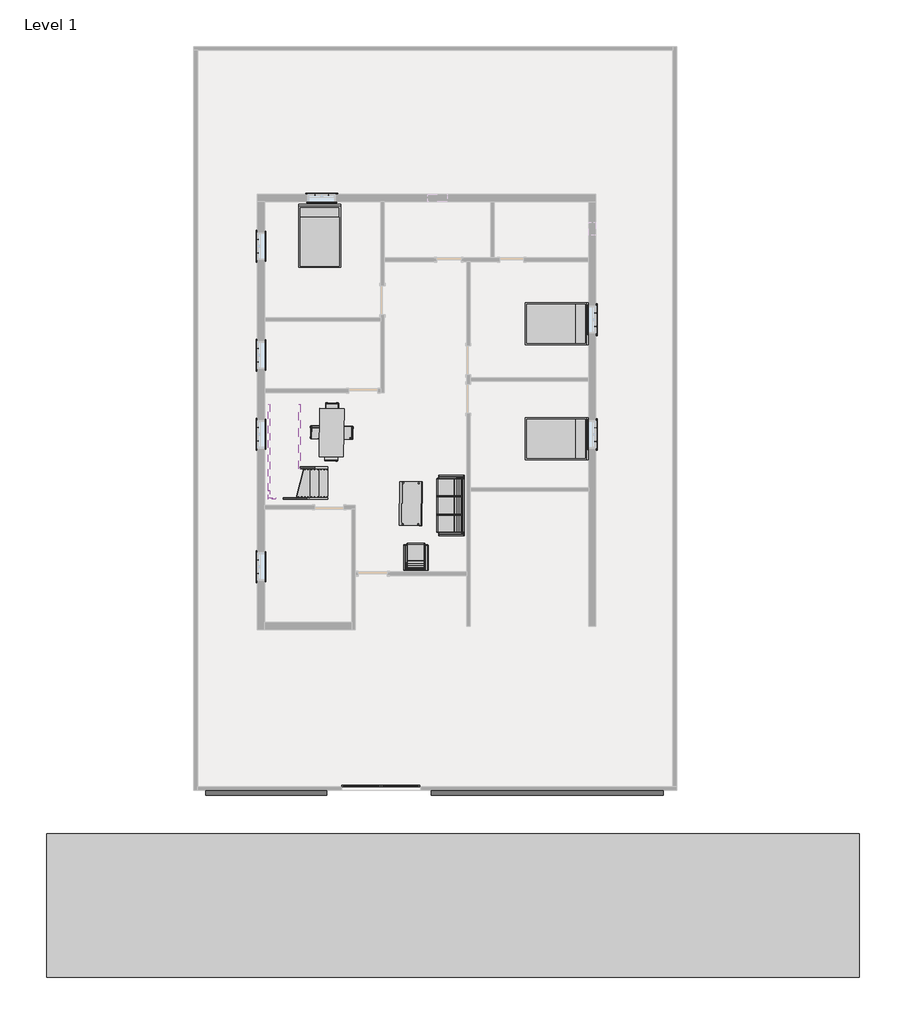
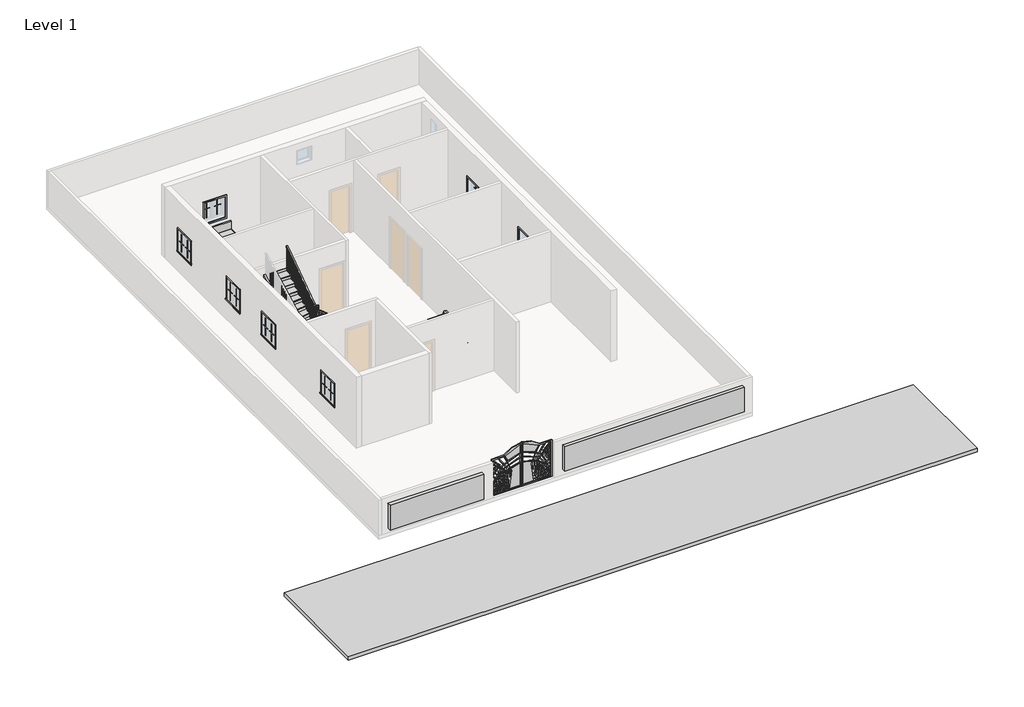
# One storey, part 2 of 2: 32 proxies, 6 furniture elements, 6 members, 1 railing, 1 stair flight.
"""IFC4 building model written with IfcOpenShell, lengths in millimetres."""

from ifc_helpers import new_model, si_unit, frame, origin, place, context, project, spatial, polyline, outline, extrude, faceted_brep, transform, mapped, element, save
from components import generic_models_6bc30956, generic_models_1_generic_models_1_70afe8e7, generic_models_2_generic_models_2_4f75562f, modern_coffee_table_17989_modern_coffee_table_17989_d3a860c8, muntin_pattern_2x2_muntin_pattern_2x2_b3fe6957, muntin_pattern_2x2_muntin_pattern_2x2_3e0ecaf2, trim_window_exterior_flat_with_sill_41619996, trim_window_interior_flat_picture_frame_51c85655, furniture_2fc85b74, furniture_29a9adb8, furniture_57072a26, furniture_f28dd14e, furniture_402a1f5e, bed_17739_bed_17739_15c61121, dining_table_w_chairs_11374_0cdfc61b, stair_flight_c47d8ec9

model = new_model("IFC4")

# Units and contexts
model_context = context("Model", 3, world=origin())
ifc_project = project(units=[si_unit("LENGTHUNIT", "METRE", prefix="MILLI")], contexts=[model_context])

# Site, building, storey
site = spatial("IfcSite", under=ifc_project)
building = spatial("IfcBuilding", under=site)
storey = spatial("IfcBuildingStorey", under=building, Name="Level 1", Elevation=0.0)

# Proxies
placement = place(None, origin())
generic_models_shape = generic_models_6bc30956(model_context)
element("IfcBuildingElementProxy", 1, Name="Generic Models", at=placement, inside=storey, context=model_context, shape_type="MappedRepresentation", body=[
    mapped(generic_models_shape, transform((-2704.2599931, -11222.4732708, 0.0), x_axis=(1.0, 0.0, 0.0), y_axis=(0.0, 1.0, 0.0), z_axis=(0.0, 0.0, 1.0))),
])
generic_models_1_generic_models_1_shape = generic_models_1_generic_models_1_70afe8e7(model_context)
element("IfcBuildingElementProxy", 2, Name="Generic Models 1 : Generic Models 1", ObjectType="Generic Models 1 : Generic Models 1", at=placement, inside=storey, context=model_context, shape_type="MappedRepresentation", body=[
    mapped(generic_models_1_generic_models_1_shape, transform((0.0, 0.0, 0.0), x_axis=(1.0, 0.0, 0.0), y_axis=(0.0, 1.0, 0.0), z_axis=(0.0, 0.0, 1.0))),
])
generic_models_2_generic_models_2_shape = generic_models_2_generic_models_2_4f75562f(model_context)
element("IfcBuildingElementProxy", 3, Name="Generic Models 2 : Generic Models 2", ObjectType="Generic Models 2 : Generic Models 2", at=placement, inside=storey, context=model_context, shape_type="MappedRepresentation", body=[
    mapped(generic_models_2_generic_models_2_shape, transform((0.0, 0.0, 0.0), x_axis=(1.0, 0.0, 0.0), y_axis=(0.0, 1.0, 0.0), z_axis=(0.0, 0.0, 1.0))),
])
modern_coffee_table_17989_modern_coffee_table_17989_shape = modern_coffee_table_17989_modern_coffee_table_17989_d3a860c8(model_context)
element("IfcBuildingElementProxy", 4, Name="Modern_Coffee_Table_17989 : Modern_Coffee_Table_17989", ObjectType="Modern_Coffee_Table_17989 : Modern_Coffee_Table_17989", at=placement, inside=storey, context=model_context, shape_type="MappedRepresentation", body=[
    mapped(modern_coffee_table_17989_modern_coffee_table_17989_shape, transform((-2106.8718825, -2116.758017, 0.0), x_axis=(0.012591066442684793, 0.9999207293810025, 0.0), y_axis=(-0.9999207293810025, 0.012591066442684793, 0.0), z_axis=(0.0, 0.0, 1.0))),
])
muntin_pattern_2x2_muntin_pattern_2x2_shape = muntin_pattern_2x2_muntin_pattern_2x2_b3fe6957(model_context)
element("IfcBuildingElementProxy", 5, Name="Muntin Pattern_2x2 : Muntin Pattern_2x2", ObjectType="Muntin Pattern_2x2 : Muntin Pattern_2x2", at=placement, inside=storey, context=model_context, shape_type="MappedRepresentation", body=[
    mapped(muntin_pattern_2x2_muntin_pattern_2x2_shape, transform((-4775.9474931, 7386.6685985, 984.25), x_axis=(1.0, 0.0, 0.0), y_axis=(0.0, 1.0, 0.0), z_axis=(0.0, 0.0, 1.0))),
])
element("IfcBuildingElementProxy", 6, Name="Muntin Pattern_2x2 : Muntin Pattern_2x2", ObjectType="Muntin Pattern_2x2 : Muntin Pattern_2x2", at=placement, inside=storey, context=model_context, shape_type="MappedRepresentation", body=[
    mapped(muntin_pattern_2x2_muntin_pattern_2x2_shape, transform((4068.0150069, 3660.8060985, 984.25), x_axis=(0.0, -1.0, 0.0), y_axis=(1.0, 0.0, 0.0), z_axis=(0.0, 0.0, 1.0))),
])
element("IfcBuildingElementProxy", 7, Name="Muntin Pattern_2x2 : Muntin Pattern_2x2", ObjectType="Muntin Pattern_2x2 : Muntin Pattern_2x2", at=placement, inside=storey, context=model_context, shape_type="MappedRepresentation", body=[
    mapped(muntin_pattern_2x2_muntin_pattern_2x2_shape, transform((4068.0150069, 40.9802908, 984.25), x_axis=(0.0, -1.0, 0.0), y_axis=(1.0, 0.0, 0.0), z_axis=(0.0, 0.0, 1.0))),
])
element("IfcBuildingElementProxy", 8, Name="Muntin Pattern_2x2 : Muntin Pattern_2x2", ObjectType="Muntin Pattern_2x2 : Muntin Pattern_2x2", at=placement, inside=storey, context=model_context, shape_type="MappedRepresentation", body=[
    mapped(muntin_pattern_2x2_muntin_pattern_2x2_shape, transform((-6580.9349931, 2114.5810985, 984.25), x_axis=(0.0, 1.0, 0.0), y_axis=(-1.0, 0.0, 0.0), z_axis=(0.0, 0.0, 1.0))),
])
element("IfcBuildingElementProxy", 9, Name="Muntin Pattern_2x2 : Muntin Pattern_2x2", ObjectType="Muntin Pattern_2x2 : Muntin Pattern_2x2", at=placement, inside=storey, context=model_context, shape_type="MappedRepresentation", body=[
    mapped(muntin_pattern_2x2_muntin_pattern_2x2_shape, transform((-6580.9349931, 5543.5810985, 984.25), x_axis=(0.0, 1.0, 0.0), y_axis=(-1.0, 0.0, 0.0), z_axis=(0.0, 0.0, 1.0))),
])
element("IfcBuildingElementProxy", 10, Name="Muntin Pattern_2x2 : Muntin Pattern_2x2", ObjectType="Muntin Pattern_2x2 : Muntin Pattern_2x2", at=placement, inside=storey, context=model_context, shape_type="MappedRepresentation", body=[
    mapped(muntin_pattern_2x2_muntin_pattern_2x2_shape, transform((-6580.9349931, -4549.7439015, 984.25), x_axis=(0.0, 1.0, 0.0), y_axis=(-1.0, 0.0, 0.0), z_axis=(0.0, 0.0, 1.0))),
])
element("IfcBuildingElementProxy", 11, Name="Muntin Pattern_2x2 : Muntin Pattern_2x2", ObjectType="Muntin Pattern_2x2 : Muntin Pattern_2x2", at=placement, inside=storey, context=model_context, shape_type="MappedRepresentation", body=[
    mapped(muntin_pattern_2x2_muntin_pattern_2x2_shape, transform((-6580.9349931, -380.9689015, 984.25), x_axis=(0.0, 1.0, 0.0), y_axis=(-1.0, 0.0, 0.0), z_axis=(0.0, 0.0, 1.0))),
])
muntin_pattern_2x2_muntin_pattern_2x2_2_shape = muntin_pattern_2x2_muntin_pattern_2x2_3e0ecaf2(model_context)
element("IfcBuildingElementProxy", 12, Name="Muntin Pattern_2x2 : Muntin Pattern_2x2", ObjectType="Muntin Pattern_2x2 : Muntin Pattern_2x2", at=placement, inside=storey, context=model_context, shape_type="MappedRepresentation", body=[
    mapped(muntin_pattern_2x2_muntin_pattern_2x2_2_shape, transform((-4347.3224931, 7386.6685985, 984.25), x_axis=(-1.0, 0.0, 0.0), y_axis=(0.0, -1.0, 0.0), z_axis=(0.0, 0.0, 1.0))),
])
element("IfcBuildingElementProxy", 13, Name="Muntin Pattern_2x2 : Muntin Pattern_2x2", ObjectType="Muntin Pattern_2x2 : Muntin Pattern_2x2", at=placement, inside=storey, context=model_context, shape_type="MappedRepresentation", body=[
    mapped(muntin_pattern_2x2_muntin_pattern_2x2_2_shape, transform((4068.0150069, 3232.1810985, 984.25), x_axis=(0.0, 1.0, 0.0), y_axis=(-1.0, 0.0, 0.0), z_axis=(0.0, 0.0, 1.0))),
])
element("IfcBuildingElementProxy", 14, Name="Muntin Pattern_2x2 : Muntin Pattern_2x2", ObjectType="Muntin Pattern_2x2 : Muntin Pattern_2x2", at=placement, inside=storey, context=model_context, shape_type="MappedRepresentation", body=[
    mapped(muntin_pattern_2x2_muntin_pattern_2x2_2_shape, transform((4068.0150069, -387.6447092, 984.25), x_axis=(0.0, 1.0, 0.0), y_axis=(-1.0, 0.0, 0.0), z_axis=(0.0, 0.0, 1.0))),
])
element("IfcBuildingElementProxy", 15, Name="Muntin Pattern_2x2 : Muntin Pattern_2x2", ObjectType="Muntin Pattern_2x2 : Muntin Pattern_2x2", at=placement, inside=storey, context=model_context, shape_type="MappedRepresentation", body=[
    mapped(muntin_pattern_2x2_muntin_pattern_2x2_2_shape, transform((-6580.9349931, 2543.2060985, 984.25), x_axis=(0.0, -1.0, 0.0), y_axis=(1.0, 0.0, 0.0), z_axis=(0.0, 0.0, 1.0))),
])
element("IfcBuildingElementProxy", 16, Name="Muntin Pattern_2x2 : Muntin Pattern_2x2", ObjectType="Muntin Pattern_2x2 : Muntin Pattern_2x2", at=placement, inside=storey, context=model_context, shape_type="MappedRepresentation", body=[
    mapped(muntin_pattern_2x2_muntin_pattern_2x2_2_shape, transform((-6580.9349931, 5972.2060985, 984.25), x_axis=(0.0, -1.0, 0.0), y_axis=(1.0, 0.0, 0.0), z_axis=(0.0, 0.0, 1.0))),
])
element("IfcBuildingElementProxy", 17, Name="Muntin Pattern_2x2 : Muntin Pattern_2x2", ObjectType="Muntin Pattern_2x2 : Muntin Pattern_2x2", at=placement, inside=storey, context=model_context, shape_type="MappedRepresentation", body=[
    mapped(muntin_pattern_2x2_muntin_pattern_2x2_2_shape, transform((-6580.9349931, -4121.1189015, 984.25), x_axis=(0.0, -1.0, 0.0), y_axis=(1.0, 0.0, 0.0), z_axis=(0.0, 0.0, 1.0))),
])
element("IfcBuildingElementProxy", 18, Name="Muntin Pattern_2x2 : Muntin Pattern_2x2", ObjectType="Muntin Pattern_2x2 : Muntin Pattern_2x2", at=placement, inside=storey, context=model_context, shape_type="MappedRepresentation", body=[
    mapped(muntin_pattern_2x2_muntin_pattern_2x2_2_shape, transform((-6580.9349931, 47.6560985, 984.25), x_axis=(0.0, -1.0, 0.0), y_axis=(1.0, 0.0, 0.0), z_axis=(0.0, 0.0, 1.0))),
])
trim_window_exterior_flat_with_sill_shape = trim_window_exterior_flat_with_sill_41619996(model_context)
element("IfcBuildingElementProxy", 19, Name="Trim-Window-Exterior-Flat : with Sill", ObjectType="Trim-Window-Exterior-Flat : with Sill", at=placement, inside=storey, context=model_context, shape_type="MappedRepresentation", body=[
    mapped(trim_window_exterior_flat_with_sill_shape, transform((-4561.6349931, 7396.1935985, 1828.8), x_axis=(-1.0, 0.0, 0.0), y_axis=(0.0, 0.0, 1.0), z_axis=(0.0, 1.0, 0.0))),
])
element("IfcBuildingElementProxy", 20, Name="Trim-Window-Exterior-Flat : with Sill", ObjectType="Trim-Window-Exterior-Flat : with Sill", at=placement, inside=storey, context=model_context, shape_type="MappedRepresentation", body=[
    mapped(trim_window_exterior_flat_with_sill_shape, transform((4077.5400069, 3446.4935985, 1828.8), x_axis=(0.0, 1.0, 0.0), y_axis=(0.0, 0.0, 1.0), z_axis=(1.0, 0.0, 0.0))),
])
element("IfcBuildingElementProxy", 21, Name="Trim-Window-Exterior-Flat : with Sill", ObjectType="Trim-Window-Exterior-Flat : with Sill", at=placement, inside=storey, context=model_context, shape_type="MappedRepresentation", body=[
    mapped(trim_window_exterior_flat_with_sill_shape, transform((4077.5400069, -173.3322092, 1828.8), x_axis=(0.0, 1.0, 0.0), y_axis=(0.0, 0.0, 1.0), z_axis=(1.0, 0.0, 0.0))),
])
element("IfcBuildingElementProxy", 22, Name="Trim-Window-Exterior-Flat : with Sill", ObjectType="Trim-Window-Exterior-Flat : with Sill", at=placement, inside=storey, context=model_context, shape_type="MappedRepresentation", body=[
    mapped(trim_window_exterior_flat_with_sill_shape, transform((-6590.4599931, 2328.8935985, 1828.8), x_axis=(0.0, -1.0, 0.0), y_axis=(0.0, 0.0, 1.0), z_axis=(-1.0, 0.0, 0.0))),
])
element("IfcBuildingElementProxy", 23, Name="Trim-Window-Exterior-Flat : with Sill", ObjectType="Trim-Window-Exterior-Flat : with Sill", at=placement, inside=storey, context=model_context, shape_type="MappedRepresentation", body=[
    mapped(trim_window_exterior_flat_with_sill_shape, transform((-6590.4599931, 5757.8935985, 1828.8), x_axis=(0.0, -1.0, 0.0), y_axis=(0.0, 0.0, 1.0), z_axis=(-1.0, 0.0, 0.0))),
])
element("IfcBuildingElementProxy", 24, Name="Trim-Window-Exterior-Flat : with Sill", ObjectType="Trim-Window-Exterior-Flat : with Sill", at=placement, inside=storey, context=model_context, shape_type="MappedRepresentation", body=[
    mapped(trim_window_exterior_flat_with_sill_shape, transform((-6590.4599931, -4335.4314015, 1828.8), x_axis=(0.0, -1.0, 0.0), y_axis=(0.0, 0.0, 1.0), z_axis=(-1.0, 0.0, 0.0))),
])
element("IfcBuildingElementProxy", 25, Name="Trim-Window-Exterior-Flat : with Sill", ObjectType="Trim-Window-Exterior-Flat : with Sill", at=placement, inside=storey, context=model_context, shape_type="MappedRepresentation", body=[
    mapped(trim_window_exterior_flat_with_sill_shape, transform((-6590.4599931, -166.6564015, 1828.8), x_axis=(0.0, -1.0, 0.0), y_axis=(0.0, 0.0, 1.0), z_axis=(-1.0, 0.0, 0.0))),
])
trim_window_interior_flat_picture_frame_shape = trim_window_interior_flat_picture_frame_51c85655(model_context)
element("IfcBuildingElementProxy", 26, Name="Trim-Window-Interior-Flat : Picture Frame", ObjectType="Trim-Window-Interior-Flat : Picture Frame", at=placement, inside=storey, context=model_context, shape_type="MappedRepresentation", body=[
    mapped(trim_window_interior_flat_picture_frame_shape, transform((-4561.6349931, 7167.5935985, 1828.8), x_axis=(1.0, 0.0, 0.0), y_axis=(0.0, 0.0, 1.0), z_axis=(0.0, -1.0, 0.0))),
])
element("IfcBuildingElementProxy", 27, Name="Trim-Window-Interior-Flat : Picture Frame", ObjectType="Trim-Window-Interior-Flat : Picture Frame", at=placement, inside=storey, context=model_context, shape_type="MappedRepresentation", body=[
    mapped(trim_window_interior_flat_picture_frame_shape, transform((3848.9400069, 3446.4935985, 1828.8), x_axis=(0.0, -1.0, 0.0), y_axis=(0.0, 0.0, 1.0), z_axis=(-1.0, 0.0, 0.0))),
])
element("IfcBuildingElementProxy", 28, Name="Trim-Window-Interior-Flat : Picture Frame", ObjectType="Trim-Window-Interior-Flat : Picture Frame", at=placement, inside=storey, context=model_context, shape_type="MappedRepresentation", body=[
    mapped(trim_window_interior_flat_picture_frame_shape, transform((3848.9400069, -173.3322092, 1828.8), x_axis=(0.0, -1.0, 0.0), y_axis=(0.0, 0.0, 1.0), z_axis=(-1.0, 0.0, 0.0))),
])
element("IfcBuildingElementProxy", 29, Name="Trim-Window-Interior-Flat : Picture Frame", ObjectType="Trim-Window-Interior-Flat : Picture Frame", at=placement, inside=storey, context=model_context, shape_type="MappedRepresentation", body=[
    mapped(trim_window_interior_flat_picture_frame_shape, transform((-6361.8599931, 2328.8935985, 1828.8), x_axis=(0.0, 1.0, 0.0), y_axis=(0.0, 0.0, 1.0), z_axis=(1.0, 0.0, 0.0))),
])
element("IfcBuildingElementProxy", 30, Name="Trim-Window-Interior-Flat : Picture Frame", ObjectType="Trim-Window-Interior-Flat : Picture Frame", at=placement, inside=storey, context=model_context, shape_type="MappedRepresentation", body=[
    mapped(trim_window_interior_flat_picture_frame_shape, transform((-6361.8599931, 5757.8935985, 1828.8), x_axis=(0.0, 1.0, 0.0), y_axis=(0.0, 0.0, 1.0), z_axis=(1.0, 0.0, 0.0))),
])
element("IfcBuildingElementProxy", 31, Name="Trim-Window-Interior-Flat : Picture Frame", ObjectType="Trim-Window-Interior-Flat : Picture Frame", at=placement, inside=storey, context=model_context, shape_type="MappedRepresentation", body=[
    mapped(trim_window_interior_flat_picture_frame_shape, transform((-6361.8599931, -4335.4314015, 1828.8), x_axis=(0.0, 1.0, 0.0), y_axis=(0.0, 0.0, 1.0), z_axis=(1.0, 0.0, 0.0))),
])
element("IfcBuildingElementProxy", 32, Name="Trim-Window-Interior-Flat : Picture Frame", ObjectType="Trim-Window-Interior-Flat : Picture Frame", at=placement, inside=storey, context=model_context, shape_type="MappedRepresentation", body=[
    mapped(trim_window_interior_flat_picture_frame_shape, transform((-6361.8599931, -166.6564015, 1828.8), x_axis=(0.0, 1.0, 0.0), y_axis=(0.0, 0.0, 1.0), z_axis=(1.0, 0.0, 0.0))),
])

# Furniture
furniture_shape = furniture_2fc85b74(model_context)
furniture_2_shape = furniture_29a9adb8(model_context)
furniture_3_shape = furniture_57072a26(model_context)
element("IfcFurniture", 33, at=placement, inside=storey, context=model_context, shape_type="MappedRepresentation", body=[
    mapped(furniture_shape, transform((-877.7263413, -2408.2064015, 0.0), x_axis=(0.0, -1.0, 0.0), y_axis=(1.0, 0.0, 0.0), z_axis=(0.0, 0.0, 1.0))),
    mapped(furniture_2_shape, transform((-877.7263413, -2408.2064015, 0.0), x_axis=(0.0, -1.0, 0.0), y_axis=(1.0, 0.0, 0.0), z_axis=(0.0, 0.0, 1.0))),
    mapped(furniture_3_shape, transform((-877.7263413, -2408.2064015, 0.0), x_axis=(0.0, -1.0, 0.0), y_axis=(1.0, 0.0, 0.0), z_axis=(0.0, 0.0, 1.0))),
])
furniture_4_shape = furniture_f28dd14e(model_context)
furniture_5_shape = furniture_402a1f5e(model_context)
element("IfcFurniture", 34, at=placement, inside=storey, context=model_context, shape_type="MappedRepresentation", body=[
    mapped(furniture_4_shape, transform((-1595.4975416, -3653.2527501, 0.0), x_axis=(-1.0, 0.0, 0.0), y_axis=(0.0, -1.0, 0.0), z_axis=(0.0, 0.0, 1.0))),
    mapped(furniture_5_shape, transform((-1595.4975416, -3653.2527501, 0.0), x_axis=(-1.0, 0.0, 0.0), y_axis=(0.0, -1.0, 0.0), z_axis=(0.0, 0.0, 1.0))),
])
bed_17739_bed_17739_shape = bed_17739_bed_17739_15c61121(model_context)
element("IfcFurniture", 35, ObjectType="Bed_17739 : Bed_17739", at=placement, inside=storey, context=model_context, shape_type="MappedRepresentation", body=[
    mapped(bed_17739_bed_17739_shape, transform((-4628.3099931, 6062.6935985, 0.0), x_axis=(1.0, 0.0, 0.0), y_axis=(0.0, 1.0, 0.0), z_axis=(0.0, 0.0, 1.0))),
])
element("IfcFurniture", 36, ObjectType="Bed_17739 : Bed_17739", at=placement, inside=storey, context=model_context, shape_type="MappedRepresentation", body=[
    mapped(bed_17739_bed_17739_shape, transform((2820.2400069, 3319.4935985, 0.0), x_axis=(0.0, -1.0, 0.0), y_axis=(1.0, 0.0, 0.0), z_axis=(0.0, 0.0, 1.0))),
])
element("IfcFurniture", 37, ObjectType="Bed_17739 : Bed_17739", at=placement, inside=storey, context=model_context, shape_type="MappedRepresentation", body=[
    mapped(bed_17739_bed_17739_shape, transform((2820.2400069, -307.008017, 0.0), x_axis=(0.0, -1.0, 0.0), y_axis=(1.0, 0.0, 0.0), z_axis=(0.0, 0.0, 1.0))),
])
dining_table_w_chairs_11374_shape = dining_table_w_chairs_11374_0cdfc61b(model_context)
element("IfcFurniture", 38, ObjectType="Dining_Table_w_Chairs_11374", at=placement, inside=storey, context=model_context, shape_type="MappedRepresentation", body=[
    mapped(dining_table_w_chairs_11374_shape, transform((-4154.6586335, -131.9172641, 0.0), x_axis=(0.015873758475140665, 0.9998740039584353, 0.0), y_axis=(-0.9998740039584353, 0.015873758475140665, 0.0), z_axis=(0.0, 0.0, 1.0))),
])

# Members
element("IfcMember", 39, ObjectType="Stringer - 2\" Width", at=placement, inside=storey, context=model_context, shape_type="SweptSolid", body=[
    extrude(outline(polyline([(590.0562463, -4378.4230036), (922.8849999, -4378.4230036), (1638.0971411, -6009.0851964), (1305.2683876, -6009.0851964), (590.0562463, -4378.4230036)])), frame((0.0, -2211.3564015, 0.0), z_axis=(0.0, 1.0, 0.0), x_axis=(0.0, 0.0, 1.0)), (0.0, 0.0, 1.0), 50.8),
])
element("IfcMember", 40, ObjectType="Stringer - 2\" Width", at=placement, inside=storey, context=model_context, shape_type="SweptSolid", body=[
    extrude(outline(polyline([(-6009.0851964, -2160.5564015), (-6009.0851964, -2211.3564015), (-6247.5599931, -2211.3564015), (-6196.7599931, -2160.5564015), (-6009.0851964, -2160.5564015)])), frame((0.0, 0.0, 1305.2683876), z_axis=(0.0, 0.0, 1.0), x_axis=(1.0, 0.0, 0.0)), (0.0, 0.0, 1.0), 332.8287535),
])
element("IfcMember", 41, ObjectType="Stringer - 2\" Width", at=placement, inside=storey, context=model_context, shape_type="SweptSolid", body=[
    extrude(outline(polyline([(-6196.7599931, -2160.5564015), (-6247.5599931, -2211.3564015), (-6247.5599931, -1942.4030584), (-6196.7599931, -1942.4030584), (-6196.7599931, -2160.5564015)])), frame((0.0, 0.0, 1305.2683876), z_axis=(0.0, 0.0, 1.0), x_axis=(1.0, 0.0, 0.0)), (0.0, 0.0, 1.0), 332.8287535),
])
element("IfcMember", 42, ObjectType="Stringer - 2\" Width", at=placement, inside=storey, context=model_context, shape_type="SweptSolid", body=[
    extrude(outline(polyline([(-1942.4030584, 1305.2683876), (-1942.4030584, 1638.0971411), (775.380588, 3053.6189504), (775.380588, 2720.7901969), (-1942.4030584, 1305.2683876)])), frame((-6247.5599931, 0.0, 0.0), z_axis=(1.0, 0.0, 0.0), x_axis=(0.0, 1.0, 0.0)), (0.0, 0.0, 1.0), 50.8),
])
element("IfcMember", 43, ObjectType="Stringer - 2\" Width", at=placement, inside=storey, context=model_context, shape_type="SweptSolid", body=[
    extrude(outline(polyline([(435.4922729, -4378.4230036), (842.634734, -4378.4230036), (1598.1690344, -5231.5599931), (1191.0265733, -5231.5599931), (435.4922729, -4378.4230036)])), frame((0.0, -1246.1564015, 0.0), z_axis=(0.0, 1.0, 0.0), x_axis=(0.0, 0.0, 1.0)), (0.0, 0.0, 1.0), 50.8),
])
element("IfcMember", 44, ObjectType="Stringer - 2\" Width", at=placement, inside=storey, context=model_context, shape_type="SweptSolid", body=[
    extrude(outline(polyline([(-1246.1564015, 1337.7212805), (-1246.1564015, 1709.9296678), (775.380588, 3126.7693854), (775.380588, 2754.5609981), (-1246.1564015, 1337.7212805)])), frame((-5282.3599931, 0.0, 0.0), z_axis=(1.0, 0.0, 0.0), x_axis=(0.0, 1.0, 0.0)), (0.0, 0.0, 1.0), 50.8),
])

# Railing
element("IfcRailing", 45, ObjectType="Handrail - Rectangular", at=placement, inside=storey, context=model_context, shape_type="SolidModel", body=[
    faceted_brep([(-4378.4230036, -1296.9564015, 1761.0666667), (-4378.4230036, -1296.9564015, 1696.1997378), (-4378.4230036, -1246.1564015, 1696.1997378), (-4378.4230036, -1246.1564015, 1761.0666667), (-5206.1599931, -1296.9564015, 2418.3201542), (-5256.9599931, -1296.9564015, 2393.790286), (-5256.9599931, -1246.1564015, 2393.790286), (-5206.1599931, -1246.1564015, 2418.3201542), (-5206.1599931, -1296.9564015, 2625.1172738), (-5256.9599931, -1296.9564015, 2574.3172738), (-5256.9599931, -1246.1564015, 2574.3172738), (-5206.1599931, -1246.1564015, 2625.1172738), (-5333.1599931, -1296.9564015, 2625.1172738), (-5333.1599931, -1296.9564015, 2574.3172738), (-5282.3599931, -1246.1564015, 2574.3172738), (-5282.3599931, -1246.1564015, 2625.1172738), (-5333.1599931, -1169.9564015, 2625.1172738), (-5333.1599931, -1154.1797661, 2574.3172738), (-5282.3599931, -1154.1797661, 2574.3172738), (-5282.3599931, -1169.9564015, 2625.1172738), (-5333.1599931, 775.380588, 3962.4), (-5282.3599931, 775.380588, 3962.4), (-5282.3599931, 775.380588, 3900.7546698), (-5333.1599931, 775.380588, 3900.7546698)], [[[0, 1, 2, 3]], [[1, 0, 4, 5]], [[2, 1, 5, 6]], [[3, 2, 6, 7]], [[0, 3, 7, 4]], [[5, 4, 8, 9]], [[6, 5, 9, 10]], [[7, 6, 10, 11]], [[4, 7, 11, 8]], [[9, 8, 12, 13]], [[10, 9, 13, 14]], [[11, 10, 14, 15]], [[8, 11, 15, 12]], [[13, 12, 16, 17]], [[14, 13, 17, 18]], [[15, 14, 18, 19]], [[12, 15, 19, 16]], [[20, 21, 22, 23]], [[17, 16, 20, 23]], [[18, 17, 23, 22]], [[19, 18, 22, 21]], [[16, 19, 21, 20]]]),
    extrude(outline(polyline([(750.9185985, 3883.9387679), (769.9685985, 3897.0343066), (769.9685985, 2878.6666667), (750.9185985, 2878.6666667), (750.9185985, 3883.9387679)])), frame((-5317.2849931, 0.0, 0.0), z_axis=(1.0, 0.0, 0.0), x_axis=(0.0, 1.0, 0.0)), (0.0, 0.0, 1.0), 19.05),
    extrude(outline(polyline([(649.3185985, 3814.0958945), (668.3685985, 3827.1914333), (668.3685985, 2878.6666667), (649.3185985, 2878.6666667), (649.3185985, 3814.0958945)])), frame((-5317.2849931, 0.0, 0.0), z_axis=(1.0, 0.0, 0.0), x_axis=(0.0, 1.0, 0.0)), (0.0, 0.0, 1.0), 19.05),
    extrude(outline(polyline([(547.7185985, 3744.2530212), (566.7685985, 3757.3485599), (566.7685985, 2878.6666667), (547.7185985, 2878.6666667), (547.7185985, 3744.2530212)])), frame((-5317.2849931, 0.0, 0.0), z_axis=(1.0, 0.0, 0.0), x_axis=(0.0, 1.0, 0.0)), (0.0, 0.0, 1.0), 19.05),
    extrude(outline(polyline([(446.1185985, 3674.4101478), (465.1685985, 3687.5056866), (465.1685985, 2709.3333333), (446.1185985, 2709.3333333), (446.1185985, 3674.4101478)])), frame((-5317.2849931, 0.0, 0.0), z_axis=(1.0, 0.0, 0.0), x_axis=(0.0, 1.0, 0.0)), (0.0, 0.0, 1.0), 19.05),
    extrude(outline(polyline([(344.5185985, 3604.5672745), (363.5685985, 3617.6628132), (363.5685985, 2709.3333333), (344.5185985, 2709.3333333), (344.5185985, 3604.5672745)])), frame((-5317.2849931, 0.0, 0.0), z_axis=(1.0, 0.0, 0.0), x_axis=(0.0, 1.0, 0.0)), (0.0, 0.0, 1.0), 19.05),
    extrude(outline(polyline([(242.9185985, 3534.7244011), (261.9685985, 3547.8199399), (261.9685985, 2709.3333333), (242.9185985, 2709.3333333), (242.9185985, 3534.7244011)])), frame((-5317.2849931, 0.0, 0.0), z_axis=(1.0, 0.0, 0.0), x_axis=(0.0, 1.0, 0.0)), (0.0, 0.0, 1.0), 19.05),
    extrude(outline(polyline([(141.3185985, 3464.8815278), (160.3685985, 3477.9770665), (160.3685985, 2540.0), (141.3185985, 2540.0), (141.3185985, 3464.8815278)])), frame((-5317.2849931, 0.0, 0.0), z_axis=(1.0, 0.0, 0.0), x_axis=(0.0, 1.0, 0.0)), (0.0, 0.0, 1.0), 19.05),
    extrude(outline(polyline([(39.7185985, 3395.0386544), (58.7685985, 3408.1341932), (58.7685985, 2540.0), (39.7185985, 2540.0), (39.7185985, 3395.0386544)])), frame((-5317.2849931, 0.0, 0.0), z_axis=(1.0, 0.0, 0.0), x_axis=(0.0, 1.0, 0.0)), (0.0, 0.0, 1.0), 19.05),
    extrude(outline(polyline([(-61.8814015, 3325.1957811), (-42.8314015, 3338.2913198), (-42.8314015, 2370.6666667), (-61.8814015, 2370.6666667), (-61.8814015, 3325.1957811)])), frame((-5317.2849931, 0.0, 0.0), z_axis=(1.0, 0.0, 0.0), x_axis=(0.0, 1.0, 0.0)), (0.0, 0.0, 1.0), 19.05),
    extrude(outline(polyline([(-163.4814015, 3255.3529077), (-144.4314015, 3268.4484465), (-144.4314015, 2370.6666667), (-163.4814015, 2370.6666667), (-163.4814015, 3255.3529077)])), frame((-5317.2849931, 0.0, 0.0), z_axis=(1.0, 0.0, 0.0), x_axis=(0.0, 1.0, 0.0)), (0.0, 0.0, 1.0), 19.05),
    extrude(outline(polyline([(-265.0814015, 3185.5100344), (-246.0314015, 3198.6055731), (-246.0314015, 2370.6666667), (-265.0814015, 2370.6666667), (-265.0814015, 3185.5100344)])), frame((-5317.2849931, 0.0, 0.0), z_axis=(1.0, 0.0, 0.0), x_axis=(0.0, 1.0, 0.0)), (0.0, 0.0, 1.0), 19.05),
    extrude(outline(polyline([(-366.6814015, 3115.667161), (-347.6314015, 3128.7626998), (-347.6314015, 2201.3333333), (-366.6814015, 2201.3333333), (-366.6814015, 3115.667161)])), frame((-5317.2849931, 0.0, 0.0), z_axis=(1.0, 0.0, 0.0), x_axis=(0.0, 1.0, 0.0)), (0.0, 0.0, 1.0), 19.05),
    extrude(outline(polyline([(-468.2814015, 3045.8242877), (-449.2314015, 3058.9198264), (-449.2314015, 2201.3333333), (-468.2814015, 2201.3333333), (-468.2814015, 3045.8242877)])), frame((-5317.2849931, 0.0, 0.0), z_axis=(1.0, 0.0, 0.0), x_axis=(0.0, 1.0, 0.0)), (0.0, 0.0, 1.0), 19.05),
    extrude(outline(polyline([(-569.8814015, 2975.9814143), (-550.8314015, 2989.0769531), (-550.8314015, 2201.3333333), (-569.8814015, 2201.3333333), (-569.8814015, 2975.9814143)])), frame((-5317.2849931, 0.0, 0.0), z_axis=(1.0, 0.0, 0.0), x_axis=(0.0, 1.0, 0.0)), (0.0, 0.0, 1.0), 19.05),
    extrude(outline(polyline([(-671.4814015, 2906.138541), (-652.4314015, 2919.2340797), (-652.4314015, 2032.0), (-671.4814015, 2032.0), (-671.4814015, 2906.138541)])), frame((-5317.2849931, 0.0, 0.0), z_axis=(1.0, 0.0, 0.0), x_axis=(0.0, 1.0, 0.0)), (0.0, 0.0, 1.0), 19.05),
    extrude(outline(polyline([(-773.0814015, 2836.2956676), (-754.0314015, 2849.3912064), (-754.0314015, 2032.0), (-773.0814015, 2032.0), (-773.0814015, 2836.2956676)])), frame((-5317.2849931, 0.0, 0.0), z_axis=(1.0, 0.0, 0.0), x_axis=(0.0, 1.0, 0.0)), (0.0, 0.0, 1.0), 19.05),
    extrude(outline(polyline([(-874.6814015, 2766.4527943), (-855.6314015, 2779.548333), (-855.6314015, 1862.6666667), (-874.6814015, 1862.6666667), (-874.6814015, 2766.4527943)])), frame((-5317.2849931, 0.0, 0.0), z_axis=(1.0, 0.0, 0.0), x_axis=(0.0, 1.0, 0.0)), (0.0, 0.0, 1.0), 19.05),
    extrude(outline(polyline([(-976.2814015, 2696.6099209), (-957.2314015, 2709.7054597), (-957.2314015, 1862.6666667), (-976.2814015, 1862.6666667), (-976.2814015, 2696.6099209)])), frame((-5317.2849931, 0.0, 0.0), z_axis=(1.0, 0.0, 0.0), x_axis=(0.0, 1.0, 0.0)), (0.0, 0.0, 1.0), 19.05),
    extrude(outline(polyline([(-1077.8814015, 2626.7670476), (-1058.8314015, 2639.8625863), (-1058.8314015, 1693.3333333), (-1077.8814015, 1693.3333333), (-1077.8814015, 2626.7670476)])), frame((-5317.2849931, 0.0, 0.0), z_axis=(1.0, 0.0, 0.0), x_axis=(0.0, 1.0, 0.0)), (0.0, 0.0, 1.0), 19.05),
    extrude(outline(polyline([(-1179.4814015, 2556.9241742), (-1160.4314015, 2570.019713), (-1160.4314015, 1693.3333333), (-1179.4814015, 1693.3333333), (-1179.4814015, 2556.9241742)])), frame((-5317.2849931, 0.0, 0.0), z_axis=(1.0, 0.0, 0.0), x_axis=(0.0, 1.0, 0.0)), (0.0, 0.0, 1.0), 19.05),
    extrude(outline(polyline([(-5283.2980036, -1262.0314015), (-5283.2980036, -1281.0814015), (-5302.3480036, -1281.0814015), (-5302.3480036, -1262.0314015), (-5283.2980036, -1262.0314015)])), frame((0.0, 0.0, 1524.0), z_axis=(0.0, 0.0, 1.0), x_axis=(1.0, 0.0, 0.0)), (0.0, 0.0, 1.0), 1050.3172738),
    extrude(outline(polyline([(2334.0295097, -5181.6980036), (2349.1559074, -5200.7480036), (1354.6666667, -5200.7480036), (1354.6666667, -5181.6980036), (2334.0295097, -5181.6980036)])), frame((0.0, -1281.0814015, 0.0), z_axis=(0.0, 1.0, 0.0), x_axis=(0.0, 0.0, 1.0)), (0.0, 0.0, 1.0), 19.05),
    extrude(outline(polyline([(2253.3553883, -5080.0980036), (2268.4817861, -5099.1480036), (1185.3333333, -5099.1480036), (1185.3333333, -5080.0980036), (2253.3553883, -5080.0980036)])), frame((0.0, -1281.0814015, 0.0), z_axis=(0.0, 1.0, 0.0), x_axis=(0.0, 0.0, 1.0)), (0.0, 0.0, 1.0), 19.05),
    extrude(outline(polyline([(2172.681267, -4978.4980036), (2187.8076647, -4997.5480036), (1185.3333333, -4997.5480036), (1185.3333333, -4978.4980036), (2172.681267, -4978.4980036)])), frame((0.0, -1281.0814015, 0.0), z_axis=(0.0, 1.0, 0.0), x_axis=(0.0, 0.0, 1.0)), (0.0, 0.0, 1.0), 19.05),
    extrude(outline(polyline([(2092.0071456, -4876.8980036), (2107.1335434, -4895.9480036), (1016.0, -4895.9480036), (1016.0, -4876.8980036), (2092.0071456, -4876.8980036)])), frame((0.0, -1281.0814015, 0.0), z_axis=(0.0, 1.0, 0.0), x_axis=(0.0, 0.0, 1.0)), (0.0, 0.0, 1.0), 19.05),
    extrude(outline(polyline([(2011.3330243, -4775.2980036), (2026.459422, -4794.3480036), (1016.0, -4794.3480036), (1016.0, -4775.2980036), (2011.3330243, -4775.2980036)])), frame((0.0, -1281.0814015, 0.0), z_axis=(0.0, 1.0, 0.0), x_axis=(0.0, 0.0, 1.0)), (0.0, 0.0, 1.0), 19.05),
    extrude(outline(polyline([(1930.6589029, -4673.6980036), (1945.7853007, -4692.7480036), (1016.0, -4692.7480036), (1016.0, -4673.6980036), (1930.6589029, -4673.6980036)])), frame((0.0, -1281.0814015, 0.0), z_axis=(0.0, 1.0, 0.0), x_axis=(0.0, 0.0, 1.0)), (0.0, 0.0, 1.0), 19.05),
    extrude(outline(polyline([(1849.9847816, -4572.0980036), (1865.1111793, -4591.1480036), (846.6666667, -4591.1480036), (846.6666667, -4572.0980036), (1849.9847816, -4572.0980036)])), frame((0.0, -1281.0814015, 0.0), z_axis=(0.0, 1.0, 0.0), x_axis=(0.0, 0.0, 1.0)), (0.0, 0.0, 1.0), 19.05),
    extrude(outline(polyline([(1769.3106602, -4470.4980036), (1784.437058, -4489.5480036), (846.6666667, -4489.5480036), (846.6666667, -4470.4980036), (1769.3106602, -4470.4980036)])), frame((0.0, -1281.0814015, 0.0), z_axis=(0.0, 1.0, 0.0), x_axis=(0.0, 0.0, 1.0)), (0.0, 0.0, 1.0), 19.05),
    extrude(outline(polyline([(-5298.2349931, -1262.0314015), (-5298.2349931, -1281.0814015), (-5317.2849931, -1281.0814015), (-5317.2849931, -1262.0314015), (-5298.2349931, -1262.0314015)])), frame((0.0, 0.0, 1524.0), z_axis=(0.0, 0.0, 1.0), x_axis=(1.0, 0.0, 0.0)), (0.0, 0.0, 1.0), 1050.3172738),
    extrude(outline(polyline([(756.330588, 3887.659131), (775.380588, 3900.7546698), (775.380588, 2878.6666667), (756.330588, 2878.6666667), (756.330588, 3887.659131)])), frame((-5317.2849931, 0.0, 0.0), z_axis=(1.0, 0.0, 0.0), x_axis=(0.0, 1.0, 0.0)), (0.0, 0.0, 1.0), 19.05),
    extrude(outline(polyline([(1696.1997378, -4378.4230036), (1711.3261355, -4397.4730036), (846.6666667, -4397.4730036), (846.6666667, -4378.4230036), (1696.1997378, -4378.4230036)])), frame((0.0, -1281.0814015, 0.0), z_axis=(0.0, 1.0, 0.0), x_axis=(0.0, 0.0, 1.0)), (0.0, 0.0, 1.0), 19.05),
])

# Stair flight
stair_flight_shape = stair_flight_c47d8ec9(model_context)
element("IfcStairFlight", 46, ObjectType="2\" Tread 1\" Nosing 1/4\" Riser", at=placement, inside=storey, context=model_context, shape_type="MappedRepresentation", body=[
    mapped(stair_flight_shape, transform((0.0, 0.0, 0.0), x_axis=(1.0, 0.0, 0.0), y_axis=(0.0, 1.0, 0.0), z_axis=(0.0, 0.0, 1.0))),
])

save(model, "model.ifc")

# Revit data of these elements
# Type
#   m.s. sheet = none
#   2" x2" pipe = none
#   1"x1"pipe = none
#   Default Elevation = 0
# Type "Modern_Coffee_Table_17989 : Modern_Coffee_Table_17989"
#   Default Elevation = 0
# Type "Muntin Pattern_2x2 : Muntin Pattern_2x2"
#   Width [instance default] = 4' - 0"
#   Thickness = 0' - 0 1/2"
#   Height [instance default] = 4' - 0"
#   Distance = 0' - 0 3/4"
#   Interior Material [instance default] = none
#   Exterior Material [instance default] = none
#   Default Elevation = 0
# Type "Trim-Window-Exterior-Flat : with Sill"
#   Trim Width = 0' - 2 1/4"
#   Trim Thickness_Picture Frame = 0' - 1 1/4"
#   Trim Thickness_with Sill = 0' - 0 3/4"
#   Sill Thickness = 0' - 1 1/4"
#   Opening Width [instance default] = 2' - 0"
#   Opening Height [instance default] = 3' - 0"
#   Default Elevation = 4' - 0"
#   Sill = yes
#   Picture Frame = no
#   Trim Material [instance default] = none
# Type "Trim-Window-Interior-Flat : Picture Frame"
#   Trim Thickness_Picture Frame = 0' - 1 1/4"
#   Trim Width = 0' - 2 1/4"
#   Trim Thickness_with Sill = 0' - 0 3/4"
#   Sill Thickness = 0' - 1 1/4"
#   Opening Width [instance default] = 2' - 0"
#   Opening Height [instance default] = 3' - 0"
#   Default Elevation = 4' - 0"
#   Sill = no
#   Picture Frame = yes
#   Trim Material [instance default] = none
# Type
#   Width [instance] = 6' - 3.19685"
#   Default Elevation = 0
# Type
#   Width [instance] = 2' - 6.31496"
#   Default Elevation = 0
# Type "Bed_17739 : Bed_17739"
#   Default Elevation = 0
# Type "Dining_Table_w_Chairs_11374"
#   Default Elevation = 0
#   Assembly Code = ""
# Type "Handrail - Rectangular"
#   Assembly Code = "C2010400"
#   built-in parameter 1008612 = 0.0416667 (stored number, unit not read)
#   built-in parameter 1008611 = 0.0416667 (stored number, unit not read)
#   built-in parameter 1008609 = 0.333333 (stored number, unit not read)
#   built-in parameter 1008604 = 0.166667 (stored number, unit not read)
#   built-in parameter 1008603 = 0.166667 (stored number, unit not read)
#   Railing Height = 3' - 0"
#   built-in parameter 1008630 = 2
#   built-in parameter 1008610 = 2
#   built-in parameter 1008618 = Baluster - Square : 3/4"
# Element 1 (IfcBuildingElementProxy)
#   Phase Created = New Construction
#   Materials on its faces: "r1"
# Element 2 (IfcBuildingElementProxy, "Generic Models 1 : Generic Models 1")
#   Phase Created = New Construction
#   Materials on its faces: "Parking Stripe"
# Element 3 (IfcBuildingElementProxy, "Generic Models 2 : Generic Models 2")
#   Phase Created = New Construction
# Element 4 (IfcBuildingElementProxy, "Modern_Coffee_Table_17989 : Modern_Coffee_Table_17989")
#   Phase Created = New Construction
#   Materials on its faces: "1 Wood", "1 Glass", "1 Metal"
# Elements 5, 6, 7, 8, 9, 10, 11, 12, 13, 14, 15, 16, 17, 18 (IfcBuildingElementProxy, "Muntin Pattern_2x2 : Muntin Pattern_2x2")
#   Width = 0' - 11 5/8"
#   Height = 2' - 6 1/2"
#   Interior Material = Wood - Stained
#   Exterior Material = Clad - White
#   Phase Created = New Construction
#   Materials on its faces: "Clad - White", "Wood - Stained"
# Elements 19, 20, 21, 22, 23, 24, 25 (IfcBuildingElementProxy, "Trim-Window-Exterior-Flat : with Sill")
#   Opening Width = 2' - 10"
#   Opening Height = 3' - 0"
#   Trim Material = Clad - White
#   Phase Created = New Construction
#   Materials on its faces: "Clad - White"
# Elements 26, 27, 28, 29, 30, 31, 32 (IfcBuildingElementProxy, "Trim-Window-Interior-Flat : Picture Frame")
#   Opening Width = 2' - 10"
#   Opening Height = 3' - 0"
#   Trim Material = Wood - Stained
#   Phase Created = New Construction
#   Materials on its faces: "Wood - Stained"
# Element 33 (IfcFurniture)
#   Width = 6' - 3.19685"
#   Phase Created = New Construction
# Element 34 (IfcFurniture)
#   Width = 2' - 6.31496"
#   Phase Created = New Construction
# Elements 35, 36, 37 (IfcFurniture, "Bed_17739 : Bed_17739")
#   Phase Created = New Construction
#   Materials on its faces: "legs", "sheets", "bed frame", "Blanket"
# Element 38 (IfcFurniture, "Dining_Table_w_Chairs_11374")
#   Phase Created = New Construction
# Elements 39, 40, 41, 42, 43, 44 (IfcMember, "Stringer - 2\" Width")
#   Phase Created = New Construction
# Element 45 (IfcRailing, "Handrail - Rectangular")
#   Phase Created = New Construction
# Element 46 (IfcStairFlight, "2\" Tread 1\" Nosing 1/4\" Riser")
#   Phase Created = New Construction
# Materials
#   "r1": class "Generic", colour RGB 120 120 120, transparency 0, Cost = 0
#   "Parking Stripe": class "Paint", colour RGB 250 250 91, transparency 0, Cost = 0
#   "1 Wood": class "Glass", colour RGB 81 52 39, transparency 0, Cost = 0
#   "1 Glass": class "Glass", colour RGB 236 240 239, transparency 0.85, Cost = 0
#   "1 Metal": class "Glass", colour RGB 244 244 244, transparency 0, Cost = 0
#   "Clad - White": class "Wood", colour RGB 242 242 238, transparency 0, Cost = 0
#   "Wood - Stained": class "Wood", colour RGB 224 178 126, transparency 0, Cost = 0
#   "legs": colour RGB 90 73 37, transparency 0, Cost = 0
#   "sheets": colour RGB 200 195 176, transparency 0, Cost = 0
#   "bed frame": colour RGB 90 73 37, transparency 0, Cost = 0
#   "Blanket": class "System", colour RGB 59 0 1, transparency 0, Cost = 0
